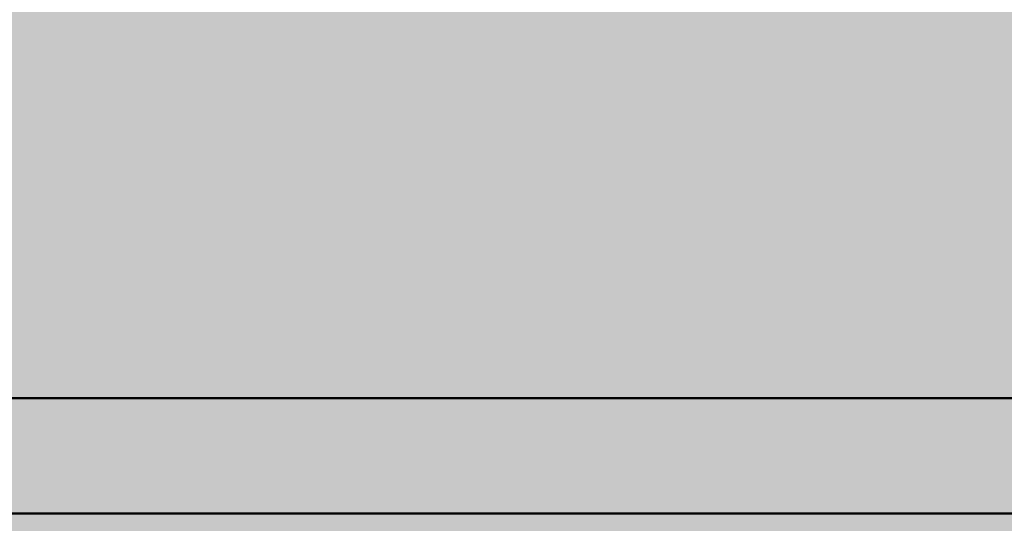
# Model space of a CAD drawing. Units: millimetres. Extents: x 0 to 2267, y 0 to 1823.
# Tile 27 of 256: x 1675 to 1760, y 1117 to 1160. Entities that reach past the tile are written whole.
import ezdxf

# ---------------------------------------------------------------- set-up
doc = ezdxf.new("R2010")
doc.units = ezdxf.units.MM
doc.header["$MEASUREMENT"] = 0
for name, color, linetype, lineweight in [('M-DIMS', 2, 'Continuous', 25), ('M-HATC', 252, 'Continuous', 18), ('M-OUTL', 7, 'Continuous', 50)]:
    doc.layers.add(name, color=color, linetype=linetype, lineweight=lineweight)
doc.styles.get("Standard").update_dxf_attribs({"font": 'arial.ttf'})
doc.dimstyles.get("Standard").update_dxf_attribs({"dimtxt": 7, "dimasz": 4, "dimexe": 0.18, "dimexo": 0.0625, "dimgap": 0.09, "dimtad": 0, "dimdec": 0, "dimzin": 0, "dimdsep": 46, "dimtxsty": 'Standard', "dimcen": 0.09, "dimadec": 0, "dimazin": 0, "dimtfac": 1, "dimtdec": 0, "dimtofl": 0, "dimtmove": 0, "dimatfit": 3, "dimfxl": 1, "dimtolj": 1, "dimtzin": 0, "dimarcsym": 0})

# ---------------------------------------------------------------- blocks, each defined once
blk = doc.blocks.new('*D1')
at = {"layer": 'Defpoints', "color": 0, "transparency": 16777216}
for p in [(1593.429, 1127.417), (1843.429, 1127.417), (1843.429, 955.628)]:
    blk.add_point(p, dxfattribs=at)
at = {"layer": 'M-DIMS', "color": 0, "lineweight": -2, "transparency": 16777216}
for p, q in [((1593.429, 1127.355), (1593.429, 955.448)), ((1843.429, 1127.355), (1843.429, 955.448)), ((1597.429, 955.628), (1710.558, 955.628)), ((1839.429, 955.628), (1726.3, 955.628))]:
    blk.add_line(p, q, dxfattribs=at)
at = {"layer": 'M-DIMS', "color": 0, "transparency": 16777216}
for points in [[(1597.429, 956.294), (1597.429, 954.961), (1593.429, 955.628)], [(1839.429, 956.294), (1839.429, 954.961), (1843.429, 955.628)]]:
    blk.add_solid(points, dxfattribs=at)
at = {"layer": 'M-DIMS', "color": 0, "transparency": 16777216, "insert": (1718.429, 955.628), "char_height": 7, "attachment_point": 5}
blk.add_mtext('\\A1;250', dxfattribs=at)

msp = doc.modelspace()

# ---------------------------------------------------------------- hatches: boundary and pattern name
at = {"layer": 'M-HATC'}
h = msp.add_hatch(color=256, dxfattribs=at)
h.dxf.hatch_style = 1
h.paths.add_polyline_path([(2065.771, 1618.062, 0.236068), (2055.771, 1638.062), (1381.087, 1638.062, 0.236068), (1371.087, 1618.062), (1371.087, 1603.062), (2055.771, 1603.062), (2065.771, 1603.062)])
h.paths.add_polyline_path([(2062.772, 1550.296), (2062.772, 1560.296), (1374.086, 1560.296), (1374.086, 1550.296), (1374.086, 1540.296), (1384.086, 1540.296), (1389.086, 1540.296), (2062.772, 1540.296)])
h.paths.add_polyline_path([(1930.929, 1282.766), (1505.929, 1282.766), (1587.628, 1235.597, 0.131652), (1600.128, 1232.247), (1836.73, 1232.247, 0.131652), (1849.23, 1235.597)])
h.paths.add_polyline_path([(1930.929, 1117.417), (1905.929, 1117.417), (1505.929, 1117.417), (1505.929, 1077.417), (1930.929, 1077.417)])
h = msp.add_hatch(color=256, dxfattribs=at)
h.dxf.hatch_style = 1
h.paths.add_polyline_path([(2055.771, 1603.062), (1381.087, 1603.062), (1381.087, 1598.062), (2055.771, 1598.062)])
h.paths.add_polyline_path([(2055.771, 1598.062), (1381.087, 1598.062), (1381.087, 1593.062), (2055.771, 1593.062)])
h.paths.add_polyline_path([(2051.307, 1536.761), (1385.55, 1536.761), (1385.55, 1526.761), (1387.55, 1526.761), (1388.537, 1525.053), (1385.332, 1521.233), (1385.332, 1521.223), (2050.254, 1522.749), (2048.321, 1525.053), (2049.307, 1526.761), (2051.307, 1526.761)])
edge = h.paths.add_edge_path()
edge.add_arc((1847.535, 1379.149), 135, 222.60306, 222.89085, ccw=False)
edge.add_line((1748.166, 1287.766), (1683.092, 1287.766))
edge.add_arc((1583.724, 1379.149), 135, 317.10915, 317.39694, ccw=False)
edge.add_arc((1678.969, 1290.671), 5, 222.89085, 317.10915, ccw=False)
edge.add_arc((1774.213, 1379.149), 135, 222.60306, 222.89085, ccw=False)
edge.add_line((1674.845, 1287.766), (1609.771, 1287.766))
edge.add_arc((1510.403, 1379.149), 135, 317.10915, 317.39694, ccw=False)
edge.add_arc((1605.647, 1290.671), 5, 222.89085, 317.10915, ccw=False)
edge.add_arc((1700.892, 1379.149), 135, 222.60306, 222.89085, ccw=False)
edge.add_line((1601.524, 1287.766), (1536.45, 1287.766))
edge.add_arc((1437.081, 1379.149), 135, 317.10915, 317.39694, ccw=False)
edge.add_arc((1532.326, 1290.671), 5, 222.89085, 317.10915, ccw=False)
edge.add_arc((1627.571, 1379.149), 135, 222.60306, 222.89085, ccw=False)
edge.add_line((1528.203, 1287.766), (1505.929, 1287.766))
edge.add_spline(control_points=[(1505.929, 1287.766), (1504.262, 1287.766), (1504.262, 1282.766), (1505.929, 1282.766)], knot_values=[0, 0, 0, 0, 5, 5, 5, 5], degree=3, periodic=0)
edge.add_line((1505.929, 1282.766), (1930.929, 1282.766))
edge.add_spline(control_points=[(1930.929, 1282.766), (1932.596, 1282.766), (1932.596, 1287.766), (1930.929, 1287.766)], knot_values=[0, 0, 0, 0, 5, 5, 5, 5], degree=3, periodic=0)
edge.add_line((1930.929, 1287.766), (1903.056, 1287.766))
edge.add_arc((1803.688, 1379.149), 135, 317.10915, 317.39694, ccw=False)
edge.add_arc((1898.932, 1290.671), 5, 222.89085, 317.10915, ccw=False)
edge.add_arc((1994.177, 1379.149), 135, 222.60306, 222.89085, ccw=False)
edge.add_line((1894.809, 1287.766), (1829.735, 1287.766))
edge.add_arc((1730.366, 1379.149), 135, 317.10915, 317.39694, ccw=False)
edge.add_arc((1825.611, 1290.671), 5, 222.89085, 317.10915, ccw=False)
edge.add_arc((1920.856, 1379.149), 135, 222.60306, 222.89085, ccw=False)
edge.add_line((1821.487, 1287.766), (1756.413, 1287.766))
edge.add_arc((1657.045, 1379.149), 135, 317.10915, 317.39694, ccw=False)
edge.add_arc((1752.29, 1290.671), 5, 222.89085, 317.10915, ccw=False)
edge = h.paths.add_edge_path()
edge.add_spline(control_points=[(1843.429, 1227.247), (1845.096, 1227.247), (1845.096, 1232.247), (1843.429, 1232.247)], knot_values=[0, 0, 0, 0, 5, 5, 5, 5], degree=3, periodic=0)
edge.add_line((1843.429, 1232.247), (1593.429, 1232.247))
edge.add_spline(control_points=[(1593.429, 1232.247), (1591.762, 1232.247), (1591.762, 1227.247), (1593.429, 1227.247)], knot_values=[0, 0, 0, 0, 5, 5, 5, 5], degree=3, periodic=0)
edge.add_line((1593.429, 1227.247), (1843.429, 1227.247))
h.paths.add_polyline_path([(1905.929, 1127.417), (1530.929, 1127.417, 0.414214), (1520.929, 1117.417), (1530.929, 1117.417), (1915.929, 1117.417, 0.414214)])
edge = h.paths.add_edge_path()
edge.add_arc((1397.086, 1498.408), 12.73, 90.78215, 190.87871, ccw=False)
edge.add_line((1396.912, 1511.136), (1428.01, 1511.349))
edge.add_line((1428.01, 1511.349), (1433.01, 1511.349))
edge.add_line((1433.01, 1511.349), (1434.439, 1511.349))
edge.add_arc((1419.474, 1498.08), 20, 41.561, 74.08211)
edge.add_line((1424.959, 1517.314), (1399.935, 1517.256))
edge.add_spline(control_points=[(1399.931, 1517.256), (1399.884, 1517.213), (1399.833, 1517.169), (1399.777, 1517.124)], knot_values=[11.567499, 11.567499, 11.567499, 11.567499, 11.814249, 11.814249, 11.814249, 11.814249], degree=3, periodic=0)
edge.add_spline(control_points=[(1399.633, 1517.01), (1399.583, 1516.972), (1399.531, 1516.934), (1399.476, 1516.895)], knot_values=[11.167718, 11.167718, 11.167718, 11.167718, 11.365188, 11.365188, 11.365188, 11.365188], degree=3, periodic=0)
edge.add_spline(control_points=[(1399.34, 1516.8), (1399.151, 1516.672), (1398.938, 1516.538), (1398.704, 1516.399)], knot_values=[10.376405, 10.376405, 10.376405, 10.376405, 11.00994, 11.00994, 11.00994, 11.00994], degree=3, periodic=0)
edge.add_spline(control_points=[(1398.657, 1516.372), (1398.579, 1516.326), (1398.498, 1516.28), (1398.415, 1516.233)], knot_values=[10.125175, 10.125175, 10.125175, 10.125175, 10.334406, 10.334406, 10.334406, 10.334406], degree=3, periodic=0)
edge.add_spline(control_points=[(1398.264, 1516.149), (1398.196, 1516.111), (1398.126, 1516.073), (1398.055, 1516.035)], knot_values=[9.832246, 9.832246, 9.832246, 9.832246, 9.999658, 9.999658, 9.999658, 9.999658], degree=3, periodic=0)
edge.add_spline(control_points=[(1397.999, 1516.005), (1397.731, 1515.862), (1397.446, 1515.717), (1397.147, 1515.571)], knot_values=[9.161808, 9.161808, 9.161808, 9.161808, 9.787769, 9.787769, 9.787769, 9.787769], degree=3, periodic=0)
edge.add_spline(control_points=[(1397.147, 1515.571), (1396.842, 1515.423), (1396.522, 1515.274), (1396.191, 1515.126)], knot_values=[8.524455, 8.524455, 8.524455, 8.524455, 9.161808, 9.161808, 9.161808, 9.161808], degree=3, periodic=0)
edge.add_spline(control_points=[(1396.078, 1515.076), (1395.985, 1515.035), (1395.892, 1514.994), (1395.798, 1514.953)], knot_values=[8.275193, 8.275193, 8.275193, 8.275193, 8.451726, 8.451726, 8.451726, 8.451726], degree=3, periodic=0)
edge.add_spline(control_points=[(1395.602, 1514.869), (1395.5, 1514.826), (1395.397, 1514.782), (1395.293, 1514.739)], knot_values=[7.962917, 7.962917, 7.962917, 7.962917, 8.152764, 8.152764, 8.152764, 8.152764], degree=3, periodic=0)
edge.add_spline(control_points=[(1395.212, 1514.706), (1394.828, 1514.547), (1394.435, 1514.393), (1394.036, 1514.244)], knot_values=[7.21254, 7.21254, 7.21254, 7.21254, 7.913148, 7.913148, 7.913148, 7.913148], degree=3, periodic=0)
edge.add_spline(control_points=[(1394.036, 1514.244), (1393.708, 1514.121), (1393.375, 1514.003), (1393.043, 1513.889)], knot_values=[6.633733, 6.633733, 6.633733, 6.633733, 7.21254, 7.21254, 7.21254, 7.21254], degree=3, periodic=0)
edge.add_spline(control_points=[(1392.821, 1513.815), (1392.72, 1513.781), (1392.618, 1513.748), (1392.517, 1513.715)], knot_values=[6.328796, 6.328796, 6.328796, 6.328796, 6.505493, 6.505493, 6.505493, 6.505493], degree=3, periodic=0)
edge.add_spline(control_points=[(1392.517, 1513.715), (1392.319, 1513.652), (1392.121, 1513.59), (1391.924, 1513.531)], knot_values=[5.984605, 5.984605, 5.984605, 5.984605, 6.328796, 6.328796, 6.328796, 6.328796], degree=3, periodic=0)
edge.add_spline(control_points=[(1391.792, 1513.491), (1391.312, 1513.35), (1390.838, 1513.224), (1390.378, 1513.117)], knot_values=[5.066697, 5.066697, 5.066697, 5.066697, 5.907055, 5.907055, 5.907055, 5.907055], degree=3, periodic=0)
edge.add_spline(control_points=[(1390.378, 1513.117), (1390.18, 1513.071), (1389.984, 1513.028), (1389.791, 1512.99)], knot_values=[4.70367, 4.70367, 4.70367, 4.70367, 5.066695, 5.066695, 5.066695, 5.066695], degree=3, periodic=0)
edge.add_spline(control_points=[(1389.422, 1512.92), (1389.246, 1512.889), (1389.073, 1512.862), (1388.904, 1512.838)], knot_values=[4.130571, 4.130571, 4.130571, 4.130571, 4.469816, 4.469816, 4.469816, 4.469816], degree=3, periodic=0)
edge.add_spline(control_points=[(1388.904, 1512.838), (1388.591, 1512.795), (1388.291, 1512.764), (1388.007, 1512.749)], knot_values=[3.504031, 3.504031, 3.504031, 3.504031, 4.130571, 4.130571, 4.130571, 4.130571], degree=3, periodic=0)
edge.add_spline(control_points=[(1387.936, 1512.746), (1387.854, 1512.742), (1387.773, 1512.74), (1387.694, 1512.739)], knot_values=[3.268866, 3.268866, 3.268866, 3.268866, 3.451164, 3.451164, 3.451164, 3.451164], degree=3, periodic=0)
edge.add_spline(control_points=[(1387.335, 1512.744), (1387.208, 1512.75), (1387.085, 1512.76), (1386.967, 1512.774)], knot_values=[2.670686, 2.670686, 2.670686, 2.670686, 2.984, 2.984, 2.984, 2.984], degree=3, periodic=0)
edge.add_spline(control_points=[(1386.833, 1512.792), (1386.821, 1512.794), (1386.809, 1512.796), (1386.797, 1512.798)], knot_values=[2.516981, 2.516981, 2.516981, 2.516981, 2.549528, 2.549528, 2.549528, 2.549528], degree=3, periodic=0)
edge.add_spline(control_points=[(1386.453, 1512.873), (1386.426, 1512.881), (1386.399, 1512.889), (1386.373, 1512.897)], knot_values=[2.095869, 2.095869, 2.095869, 2.095869, 2.17941, 2.17941, 2.17941, 2.17941], degree=3, periodic=0)
edge.add_spline(control_points=[(1386.069, 1513.019), (1386.063, 1513.022), (1386.058, 1513.025), (1386.052, 1513.028)], knot_values=[1.72453, 1.72453, 1.72453, 1.72453, 1.745933, 1.745933, 1.745933, 1.745933], degree=3, periodic=0)
edge.add_arc((1399.474, 1498.08), 20, 131.82432, 180)
edge.add_arc((1630.334, 1505.548), 250.971, 181.70518, 236.42798)
edge.add_arc((1605.34, 1483.304), 218.782, 238.66083, 243.34961)
edge.add_arc((1647.091, 1510.359), 262.899, 183.12984, 237.85344, ccw=False)
h.paths.add_polyline_path([(1406.537, 1391.964, 0.149382), (1491.551, 1296.442, -0.129517)], flags=17)
edge = h.paths.add_edge_path()
edge.add_arc((2037.384, 1498.08), 20, 0, 48.26587)
edge.add_spline(control_points=[(2050.697, 1513.005), (2050.651, 1512.985), (2050.603, 1512.966), (2050.554, 1512.948)], knot_values=[1.835652, 1.835652, 1.835652, 1.835652, 2.000781, 2.000781, 2.000781, 2.000781], degree=3, periodic=0)
edge.add_spline(control_points=[(2050.462, 1512.917), (2050.479, 1512.922), (2050.496, 1512.928), (2050.513, 1512.934)], knot_values=[2.045477, 2.045477, 2.045477, 2.045477, 2.101389, 2.101389, 2.101389, 2.101389], degree=3, periodic=0)
edge.add_spline(control_points=[(2050.129, 1512.834), (2050.198, 1512.847), (2050.266, 1512.862), (2050.331, 1512.879)], knot_values=[2.237629, 2.237629, 2.237629, 2.237629, 2.435841, 2.435841, 2.435841, 2.435841], degree=3, periodic=0)
edge.add_spline(control_points=[(2050.095, 1512.828), (2050.106, 1512.83), (2050.118, 1512.832), (2050.129, 1512.834)], knot_values=[2.435841, 2.435841, 2.435841, 2.435841, 2.468321, 2.468321, 2.468321, 2.468321], degree=3, periodic=0)
edge.add_spline(control_points=[(2049.784, 1512.785), (2049.855, 1512.792), (2049.924, 1512.801), (2049.992, 1512.811)], knot_values=[2.563852, 2.563852, 2.563852, 2.563852, 2.748541, 2.748541, 2.748541, 2.748541], degree=3, periodic=0)
edge.add_spline(control_points=[(2049.405, 1512.762), (2049.536, 1512.765), (2049.663, 1512.773), (2049.784, 1512.785)], knot_values=[2.748541, 2.748541, 2.748541, 2.748541, 3.064882, 3.064882, 3.064882, 3.064882], degree=3, periodic=0)
edge.add_spline(control_points=[(2049.17, 1512.76), (2049.234, 1512.759), (2049.297, 1512.759), (2049.358, 1512.761)], knot_values=[3.102309, 3.102309, 3.102309, 3.102309, 3.2503, 3.2503, 3.2503, 3.2503], degree=3, periodic=0)
edge.add_spline(control_points=[(2048.857, 1512.769), (2048.964, 1512.764), (2049.068, 1512.761), (2049.17, 1512.76)], knot_values=[3.2503, 3.2503, 3.2503, 3.2503, 3.486069, 3.486069, 3.486069, 3.486069], degree=3, periodic=0)
edge.add_spline(control_points=[(2048.692, 1512.779), (2048.373, 1512.801), (2048.035, 1512.841), (2047.682, 1512.897)], knot_values=[3.606429, 3.606429, 3.606429, 3.606429, 4.2989, 4.2989, 4.2989, 4.2989], degree=3, periodic=0)
edge.add_spline(control_points=[(2047.682, 1512.897), (2047.546, 1512.919), (2047.408, 1512.942), (2047.268, 1512.969)], knot_values=[4.2989, 4.2989, 4.2989, 4.2989, 4.565769, 4.565769, 4.565769, 4.565769], degree=3, periodic=0)
edge.add_spline(control_points=[(2047.268, 1512.969), (2047.145, 1512.991), (2047.021, 1513.016), (2046.895, 1513.042)], knot_values=[4.565769, 4.565769, 4.565769, 4.565769, 4.799971, 4.799971, 4.799971, 4.799971], degree=3, periodic=0)
edge.add_spline(control_points=[(2046.895, 1513.042), (2046.529, 1513.119), (2046.151, 1513.209), (2045.768, 1513.311)], knot_values=[4.799971, 4.799971, 4.799971, 4.799971, 5.483718, 5.483718, 5.483718, 5.483718], degree=3, periodic=0)
edge.add_spline(control_points=[(2045.768, 1513.311), (2045.372, 1513.415), (2044.97, 1513.532), (2044.566, 1513.659)], knot_values=[5.483718, 5.483718, 5.483718, 5.483718, 6.187866, 6.187866, 6.187866, 6.187866], degree=3, periodic=0)
edge.add_spline(control_points=[(2044.566, 1513.659), (2044.415, 1513.706), (2044.263, 1513.755), (2044.112, 1513.805)], knot_values=[6.187866, 6.187866, 6.187866, 6.187866, 6.451551, 6.451551, 6.451551, 6.451551], degree=3, periodic=0)
edge.add_spline(control_points=[(2044.112, 1513.805), (2043.997, 1513.843), (2043.882, 1513.881), (2043.767, 1513.92)], knot_values=[6.451551, 6.451551, 6.451551, 6.451551, 6.651434, 6.651434, 6.651434, 6.651434], degree=3, periodic=0)
edge.add_spline(control_points=[(2043.767, 1513.92), (2043.372, 1514.055), (2042.977, 1514.198), (2042.589, 1514.346)], knot_values=[6.651434, 6.651434, 6.651434, 6.651434, 7.338879, 7.338879, 7.338879, 7.338879], degree=3, periodic=0)
edge.add_spline(control_points=[(2042.589, 1514.346), (2042.164, 1514.507), (2041.746, 1514.675), (2041.341, 1514.846)], knot_values=[7.338879, 7.338879, 7.338879, 7.338879, 8.089209, 8.089209, 8.089209, 8.089209], degree=3, periodic=0)
edge.add_spline(control_points=[(2041.341, 1514.846), (2041.103, 1514.946), (2040.869, 1515.048), (2040.64, 1515.15)], knot_values=[8.089209, 8.089209, 8.089209, 8.089209, 8.529587, 8.529587, 8.529587, 8.529587], degree=3, periodic=0)
edge.add_spline(control_points=[(2040.51, 1515.209), (2040.082, 1515.402), (2039.675, 1515.597), (2039.295, 1515.789)], knot_values=[8.613818, 8.613818, 8.613818, 8.613818, 9.44571, 9.44571, 9.44571, 9.44571], degree=3, periodic=0)
edge.add_spline(control_points=[(2039.295, 1515.789), (2039.062, 1515.907), (2038.839, 1516.025), (2038.629, 1516.14)], knot_values=[9.44571, 9.44571, 9.44571, 9.44571, 9.956404, 9.956404, 9.956404, 9.956404], degree=3, periodic=0)
edge.add_spline(control_points=[(2038.629, 1516.14), (2038.519, 1516.2), (2038.412, 1516.26), (2038.309, 1516.319)], knot_values=[9.956404, 9.956404, 9.956404, 9.956404, 10.223542, 10.223542, 10.223542, 10.223542], degree=3, periodic=0)
edge.add_spline(control_points=[(2038.309, 1516.319), (2038.214, 1516.374), (2038.122, 1516.428), (2038.033, 1516.481)], knot_values=[10.223542, 10.223542, 10.223542, 10.223542, 10.47051, 10.47051, 10.47051, 10.47051], degree=3, periodic=0)
edge.add_spline(control_points=[(2038.033, 1516.481), (2037.786, 1516.63), (2037.564, 1516.773), (2037.372, 1516.909)], knot_values=[10.47051, 10.47051, 10.47051, 10.47051, 11.15767, 11.15767, 11.15767, 11.15767], degree=3, periodic=0)
edge.add_spline(control_points=[(2037.372, 1516.909), (2037.279, 1516.975), (2037.193, 1517.04), (2037.114, 1517.102)], knot_values=[11.15767, 11.15767, 11.15767, 11.15767, 11.49227, 11.49227, 11.49227, 11.49227], degree=3, periodic=0)
edge.add_spline(control_points=[(2036.856, 1517.326), (2036.915, 1517.269), (2036.981, 1517.21), (2037.056, 1517.149)], knot_values=[11.577341, 11.577341, 11.577341, 11.577341, 11.91035, 11.91035, 11.91035, 11.91035], degree=3, periodic=0)
edge.add_spline(control_points=[(2036.807, 1517.375), (2036.823, 1517.359), (2036.839, 1517.342), (2036.856, 1517.326)], knot_values=[11.91035, 11.91035, 11.91035, 11.91035, 12.007402, 12.007402, 12.007402, 12.007402], degree=3, periodic=0)
edge.add_spline(control_points=[(2036.702, 1517.494), (2036.71, 1517.483), (2036.72, 1517.472), (2036.729, 1517.461)], knot_values=[12.184155, 12.184155, 12.184155, 12.184155, 12.255409, 12.255409, 12.255409, 12.255409], degree=3, periodic=0)
edge.add_spline(control_points=[(2036.616, 1517.621), (2036.62, 1517.613), (2036.624, 1517.606), (2036.629, 1517.598)], knot_values=[12.487913, 12.487913, 12.487913, 12.487913, 12.541035, 12.541035, 12.541035, 12.541035], degree=3, periodic=0)
edge.add_spline(control_points=[(2036.563, 1517.786), (2036.564, 1517.779), (2036.564, 1517.773), (2036.565, 1517.766)], knot_values=[12.911761, 12.911761, 12.911761, 12.911761, 12.968286, 12.968286, 12.968286, 12.968286], degree=3, periodic=0)
edge.add_spline(control_points=[(2036.617, 1517.93), (2036.612, 1517.926), (2036.609, 1517.921), (2036.605, 1517.916)], knot_values=[13.382527, 13.382527, 13.382527, 13.382527, 13.433791, 13.433791, 13.433791, 13.433791], degree=3, periodic=0)
edge.add_spline(control_points=[(2036.749, 1518.017), (2036.736, 1518.012), (2036.724, 1518.006), (2036.712, 1518)], knot_values=[13.726299, 13.726299, 13.726299, 13.726299, 13.809928, 13.809928, 13.809928, 13.809928], degree=3, periodic=0)
edge.add_spline(control_points=[(2036.86, 1518.053), (2036.839, 1518.047), (2036.818, 1518.042), (2036.799, 1518.035)], knot_values=[13.910887, 13.910887, 13.910887, 13.910887, 14.02153, 14.02153, 14.02153, 14.02153], degree=3, periodic=0)
edge.add_line((2036.964, 1518.08), (2032.384, 1518.08))
edge.add_line((2032.384, 1518.08), (2027.384, 1518.08))
edge.add_line((2027.384, 1518.08), (2022.384, 1518.08))
edge.add_line((2022.384, 1518.08), (2017.384, 1518.08))
edge.add_arc((2017.384, 1498.08), 20, 90, 138.439)
edge.add_line((2002.419, 1511.349), (2003.848, 1511.349))
edge.add_line((2003.848, 1511.349), (2008.848, 1511.349))
edge.add_line((2008.848, 1511.349), (2039.772, 1511.138))
edge.add_arc((2039.772, 1498.408), 12.73, -10.87871, 90, ccw=False)
edge.add_arc((1789.767, 1510.359), 262.899, 302.14656, 356.87016, ccw=False)
edge.add_arc((1831.518, 1483.304), 218.782, 296.65039, 301.33917)
edge.add_arc((1806.524, 1505.548), 250.971, 303.57202, 358.29482)
h.paths.add_polyline_path([(2030.321, 1391.964, -0.129517), (1945.307, 1296.442, 0.149382)], flags=17)
edge = h.paths.add_edge_path()
edge.add_spline(control_points=[(2037.246, 1518.082), (2037.29, 1518.081), (2037.336, 1518.08), (2037.384, 1518.08)], knot_values=[0.000012, 0.000012, 0.000012, 0.000012, 0.144754, 0.144754, 0.144754, 0.144754], degree=3, periodic=0)
edge.add_line((2037.336, 1518.08), (2037.01, 1518.08))
edge.add_spline(control_points=[(2037.01, 1518.08), (2036.982, 1518.077), (2036.956, 1518.073), (2036.931, 1518.068)], knot_values=[14.13465, 14.13465, 14.13465, 14.13465, 14.247197, 14.247197, 14.247197, 14.247197], degree=3, periodic=0)
edge.add_spline(control_points=[(2036.931, 1518.068), (2036.928, 1518.067), (2036.924, 1518.067), (2036.921, 1518.066)], knot_values=[14.118315, 14.118315, 14.118315, 14.118315, 14.13465, 14.13465, 14.13465, 14.13465], degree=3, periodic=0)
edge.add_spline(control_points=[(2036.921, 1518.066), (2036.912, 1518.064), (2036.903, 1518.063), (2036.895, 1518.061)], knot_values=[14.078086, 14.078086, 14.078086, 14.078086, 14.118315, 14.118315, 14.118315, 14.118315], degree=3, periodic=0)
edge.add_spline(control_points=[(2036.895, 1518.061), (2036.883, 1518.058), (2036.872, 1518.056), (2036.86, 1518.053)], knot_values=[14.02153, 14.02153, 14.02153, 14.02153, 14.078086, 14.078086, 14.078086, 14.078086], degree=3, periodic=0)
edge.add_spline(control_points=[(2036.86, 1518.053), (2036.839, 1518.047), (2036.818, 1518.042), (2036.799, 1518.035)], knot_values=[13.910887, 13.910887, 13.910887, 13.910887, 14.02153, 14.02153, 14.02153, 14.02153], degree=3, periodic=0)
edge.add_spline(control_points=[(2036.799, 1518.035), (2036.798, 1518.035), (2036.797, 1518.035), (2036.797, 1518.035)], knot_values=[13.906906, 13.906906, 13.906906, 13.906906, 13.910887, 13.910887, 13.910887, 13.910887], degree=3, periodic=0)
edge.add_spline(control_points=[(2036.797, 1518.035), (2036.788, 1518.032), (2036.78, 1518.029), (2036.772, 1518.026)], knot_values=[13.857826, 13.857826, 13.857826, 13.857826, 13.906906, 13.906906, 13.906906, 13.906906], degree=3, periodic=0)
edge.add_spline(control_points=[(2036.772, 1518.026), (2036.764, 1518.023), (2036.756, 1518.02), (2036.749, 1518.017)], knot_values=[13.809928, 13.809928, 13.809928, 13.809928, 13.857826, 13.857826, 13.857826, 13.857826], degree=3, periodic=0)
edge.add_spline(control_points=[(2036.749, 1518.017), (2036.736, 1518.012), (2036.724, 1518.006), (2036.712, 1518)], knot_values=[13.726299, 13.726299, 13.726299, 13.726299, 13.809928, 13.809928, 13.809928, 13.809928], degree=3, periodic=0)
edge.add_spline(control_points=[(2036.712, 1518), (2036.712, 1518), (2036.712, 1518), (2036.711, 1518)], knot_values=[13.723993, 13.723993, 13.723993, 13.723993, 13.726299, 13.726299, 13.726299, 13.726299], degree=3, periodic=0)
edge.add_spline(control_points=[(2036.711, 1518), (2036.706, 1517.997), (2036.701, 1517.994), (2036.696, 1517.992)], knot_values=[13.686536, 13.686536, 13.686536, 13.686536, 13.723993, 13.723993, 13.723993, 13.723993], degree=3, periodic=0)
edge.add_spline(control_points=[(2036.696, 1517.992), (2036.692, 1517.989), (2036.687, 1517.987), (2036.683, 1517.984)], knot_values=[13.651251, 13.651251, 13.651251, 13.651251, 13.686536, 13.686536, 13.686536, 13.686536], degree=3, periodic=0)
edge.add_spline(control_points=[(2036.683, 1517.984), (2036.676, 1517.98), (2036.67, 1517.976), (2036.664, 1517.971)], knot_values=[13.596804, 13.596804, 13.596804, 13.596804, 13.651251, 13.651251, 13.651251, 13.651251], degree=3, periodic=0)
edge.add_spline(control_points=[(2036.664, 1517.971), (2036.664, 1517.971), (2036.663, 1517.971), (2036.663, 1517.971)], knot_values=[13.593956, 13.593956, 13.593956, 13.593956, 13.596804, 13.596804, 13.596804, 13.596804], degree=3, periodic=0)
edge.add_spline(control_points=[(2036.663, 1517.971), (2036.66, 1517.969), (2036.658, 1517.967), (2036.655, 1517.965)], knot_values=[13.570322, 13.570322, 13.570322, 13.570322, 13.593956, 13.593956, 13.593956, 13.593956], degree=3, periodic=0)
edge.add_spline(control_points=[(2036.655, 1517.965), (2036.653, 1517.963), (2036.65, 1517.961), (2036.647, 1517.959)], knot_values=[13.545477, 13.545477, 13.545477, 13.545477, 13.570322, 13.570322, 13.570322, 13.570322], degree=3, periodic=0)
edge.add_spline(control_points=[(2036.647, 1517.959), (2036.647, 1517.959), (2036.647, 1517.959), (2036.647, 1517.959)], knot_values=[13.543931, 13.543931, 13.543931, 13.543931, 13.545477, 13.545477, 13.545477, 13.545477], degree=3, periodic=0)
edge.add_spline(control_points=[(2036.647, 1517.959), (2036.641, 1517.954), (2036.636, 1517.949), (2036.631, 1517.945)], knot_values=[13.488237, 13.488237, 13.488237, 13.488237, 13.543931, 13.543931, 13.543931, 13.543931], degree=3, periodic=0)
edge.add_spline(control_points=[(2036.631, 1517.945), (2036.628, 1517.942), (2036.626, 1517.94), (2036.623, 1517.937)], knot_values=[13.460307, 13.460307, 13.460307, 13.460307, 13.488237, 13.488237, 13.488237, 13.488237], degree=3, periodic=0)
edge.add_spline(control_points=[(2036.623, 1517.937), (2036.622, 1517.936), (2036.62, 1517.934), (2036.618, 1517.932)], knot_values=[13.439712, 13.439712, 13.439712, 13.439712, 13.460307, 13.460307, 13.460307, 13.460307], degree=3, periodic=0)
edge.add_spline(control_points=[(2036.618, 1517.932), (2036.618, 1517.931), (2036.617, 1517.931), (2036.617, 1517.93)], knot_values=[13.433791, 13.433791, 13.433791, 13.433791, 13.439712, 13.439712, 13.439712, 13.439712], degree=3, periodic=0)
edge.add_spline(control_points=[(2036.617, 1517.93), (2036.612, 1517.926), (2036.609, 1517.921), (2036.605, 1517.916)], knot_values=[13.382527, 13.382527, 13.382527, 13.382527, 13.433791, 13.433791, 13.433791, 13.433791], degree=3, periodic=0)
edge.add_spline(control_points=[(2036.605, 1517.916), (2036.603, 1517.913), (2036.6, 1517.91), (2036.598, 1517.907)], knot_values=[13.350017, 13.350017, 13.350017, 13.350017, 13.382527, 13.382527, 13.382527, 13.382527], degree=3, periodic=0)
edge.add_spline(control_points=[(2036.598, 1517.907), (2036.597, 1517.906), (2036.596, 1517.904), (2036.595, 1517.903)], knot_values=[13.333922, 13.333922, 13.333922, 13.333922, 13.350017, 13.350017, 13.350017, 13.350017], degree=3, periodic=0)
edge.add_spline(control_points=[(2036.595, 1517.903), (2036.595, 1517.902), (2036.594, 1517.901), (2036.593, 1517.9)], knot_values=[13.323828, 13.323828, 13.323828, 13.323828, 13.333922, 13.333922, 13.333922, 13.333922], degree=3, periodic=0)
edge.add_spline(control_points=[(2036.593, 1517.9), (2036.59, 1517.895), (2036.588, 1517.891), (2036.585, 1517.886)], knot_values=[13.277545, 13.277545, 13.277545, 13.277545, 13.323828, 13.323828, 13.323828, 13.323828], degree=3, periodic=0)
edge.add_spline(control_points=[(2036.585, 1517.886), (2036.584, 1517.883), (2036.582, 1517.879), (2036.58, 1517.875)], knot_values=[13.240119, 13.240119, 13.240119, 13.240119, 13.277545, 13.277545, 13.277545, 13.277545], degree=3, periodic=0)
edge.add_spline(control_points=[(2036.58, 1517.875), (2036.58, 1517.874), (2036.579, 1517.873), (2036.578, 1517.872)], knot_values=[13.228211, 13.228211, 13.228211, 13.228211, 13.240119, 13.240119, 13.240119, 13.240119], degree=3, periodic=0)
edge.add_spline(control_points=[(2036.578, 1517.872), (2036.578, 1517.87), (2036.577, 1517.869), (2036.577, 1517.868)], knot_values=[13.215717, 13.215717, 13.215717, 13.215717, 13.228211, 13.228211, 13.228211, 13.228211], degree=3, periodic=0)
edge.add_spline(control_points=[(2036.577, 1517.868), (2036.575, 1517.864), (2036.574, 1517.86), (2036.573, 1517.857)], knot_values=[13.179847, 13.179847, 13.179847, 13.179847, 13.215717, 13.215717, 13.215717, 13.215717], degree=3, periodic=0)
edge.add_spline(control_points=[(2036.573, 1517.857), (2036.571, 1517.851), (2036.57, 1517.846), (2036.569, 1517.841)], knot_values=[13.132017, 13.132017, 13.132017, 13.132017, 13.179847, 13.179847, 13.179847, 13.179847], degree=3, periodic=0)
edge.add_spline(control_points=[(2036.569, 1517.841), (2036.568, 1517.84), (2036.568, 1517.839), (2036.568, 1517.838)], knot_values=[13.122482, 13.122482, 13.122482, 13.122482, 13.132017, 13.132017, 13.132017, 13.132017], degree=3, periodic=0)
edge.add_spline(control_points=[(2036.568, 1517.838), (2036.568, 1517.836), (2036.567, 1517.835), (2036.567, 1517.833)], knot_values=[13.105592, 13.105592, 13.105592, 13.105592, 13.122482, 13.122482, 13.122482, 13.122482], degree=3, periodic=0)
edge.add_spline(control_points=[(2036.567, 1517.833), (2036.566, 1517.829), (2036.566, 1517.826), (2036.565, 1517.822)], knot_values=[13.074063, 13.074063, 13.074063, 13.074063, 13.105592, 13.105592, 13.105592, 13.105592], degree=3, periodic=0)
edge.add_spline(control_points=[(2036.565, 1517.822), (2036.565, 1517.822), (2036.565, 1517.822), (2036.565, 1517.822)], knot_values=[13.074043, 13.074043, 13.074043, 13.074043, 13.074063, 13.074063, 13.074063, 13.074063], degree=3, periodic=0)
edge.add_spline(control_points=[(2036.565, 1517.822), (2036.564, 1517.816), (2036.564, 1517.811), (2036.564, 1517.805)], knot_values=[13.021884, 13.021884, 13.021884, 13.021884, 13.074043, 13.074043, 13.074043, 13.074043], degree=3, periodic=0)
edge.add_spline(control_points=[(2036.564, 1517.805), (2036.564, 1517.804), (2036.564, 1517.803), (2036.564, 1517.803)], knot_values=[13.01674, 13.01674, 13.01674, 13.01674, 13.021884, 13.021884, 13.021884, 13.021884], degree=3, periodic=0)
edge.add_spline(control_points=[(2036.564, 1517.803), (2036.563, 1517.801), (2036.563, 1517.798), (2036.563, 1517.796)], knot_values=[12.996438, 12.996438, 12.996438, 12.996438, 13.01674, 13.01674, 13.01674, 13.01674], degree=3, periodic=0)
edge.add_spline(control_points=[(2036.563, 1517.796), (2036.563, 1517.793), (2036.563, 1517.789), (2036.563, 1517.786)], knot_values=[12.968286, 12.968286, 12.968286, 12.968286, 12.996438, 12.996438, 12.996438, 12.996438], degree=3, periodic=0)
edge.add_spline(control_points=[(2036.563, 1517.786), (2036.564, 1517.779), (2036.564, 1517.773), (2036.565, 1517.766)], knot_values=[12.911761, 12.911761, 12.911761, 12.911761, 12.968286, 12.968286, 12.968286, 12.968286], degree=3, periodic=0)
edge.add_spline(control_points=[(2036.565, 1517.766), (2036.565, 1517.766), (2036.565, 1517.766), (2036.565, 1517.766)], knot_values=[12.911017, 12.911017, 12.911017, 12.911017, 12.911761, 12.911761, 12.911761, 12.911761], degree=3, periodic=0)
edge.add_spline(control_points=[(2036.565, 1517.766), (2036.565, 1517.762), (2036.566, 1517.759), (2036.566, 1517.756)], knot_values=[12.88528, 12.88528, 12.88528, 12.88528, 12.911017, 12.911017, 12.911017, 12.911017], degree=3, periodic=0)
edge.add_spline(control_points=[(2036.566, 1517.756), (2036.567, 1517.753), (2036.567, 1517.751), (2036.568, 1517.748)], knot_values=[12.862519, 12.862519, 12.862519, 12.862519, 12.88528, 12.88528, 12.88528, 12.88528], degree=3, periodic=0)
edge.add_spline(control_points=[(2036.568, 1517.748), (2036.568, 1517.747), (2036.568, 1517.747), (2036.568, 1517.746)], knot_values=[12.858885, 12.858885, 12.858885, 12.858885, 12.862519, 12.862519, 12.862519, 12.862519], degree=3, periodic=0)
edge.add_spline(control_points=[(2036.568, 1517.746), (2036.569, 1517.74), (2036.571, 1517.733), (2036.572, 1517.726)], knot_values=[12.8053, 12.8053, 12.8053, 12.8053, 12.858885, 12.858885, 12.858885, 12.858885], degree=3, periodic=0)
edge.add_spline(control_points=[(2036.572, 1517.726), (2036.573, 1517.723), (2036.574, 1517.719), (2036.576, 1517.715)], knot_values=[12.775176, 12.775176, 12.775176, 12.775176, 12.8053, 12.8053, 12.8053, 12.8053], degree=3, periodic=0)
edge.add_spline(control_points=[(2036.576, 1517.715), (2036.576, 1517.713), (2036.577, 1517.71), (2036.578, 1517.708)], knot_values=[12.756759, 12.756759, 12.756759, 12.756759, 12.775176, 12.775176, 12.775176, 12.775176], degree=3, periodic=0)
edge.add_spline(control_points=[(2036.578, 1517.708), (2036.578, 1517.707), (2036.578, 1517.706), (2036.579, 1517.705)], knot_values=[12.748742, 12.748742, 12.748742, 12.748742, 12.756759, 12.756759, 12.756759, 12.756759], degree=3, periodic=0)
edge.add_spline(control_points=[(2036.579, 1517.705), (2036.581, 1517.698), (2036.583, 1517.692), (2036.586, 1517.685)], knot_values=[12.69959, 12.69959, 12.69959, 12.69959, 12.748742, 12.748742, 12.748742, 12.748742], degree=3, periodic=0)
edge.add_spline(control_points=[(2036.586, 1517.685), (2036.588, 1517.68), (2036.59, 1517.675), (2036.592, 1517.669)], knot_values=[12.659038, 12.659038, 12.659038, 12.659038, 12.69959, 12.69959, 12.69959, 12.69959], degree=3, periodic=0)
edge.add_spline(control_points=[(2036.592, 1517.669), (2036.594, 1517.665), (2036.596, 1517.66), (2036.598, 1517.656)], knot_values=[12.626806, 12.626806, 12.626806, 12.626806, 12.659038, 12.659038, 12.659038, 12.659038], degree=3, periodic=0)
edge.add_spline(control_points=[(2036.598, 1517.656), (2036.598, 1517.655), (2036.599, 1517.654), (2036.599, 1517.653)], knot_values=[12.619394, 12.619394, 12.619394, 12.619394, 12.626806, 12.626806, 12.626806, 12.626806], degree=3, periodic=0)
edge.add_spline(control_points=[(2036.599, 1517.653), (2036.604, 1517.642), (2036.61, 1517.632), (2036.616, 1517.621)], knot_values=[12.541039, 12.541039, 12.541039, 12.541039, 12.619394, 12.619394, 12.619394, 12.619394], degree=3, periodic=0)
edge.add_spline(control_points=[(2036.616, 1517.621), (2036.616, 1517.621), (2036.616, 1517.621), (2036.616, 1517.621)], knot_values=[12.541035, 12.541035, 12.541035, 12.541035, 12.541039, 12.541039, 12.541039, 12.541039], degree=3, periodic=0)
edge.add_spline(control_points=[(2036.616, 1517.621), (2036.62, 1517.613), (2036.624, 1517.606), (2036.629, 1517.598)], knot_values=[12.487913, 12.487913, 12.487913, 12.487913, 12.541035, 12.541035, 12.541035, 12.541035], degree=3, periodic=0)
edge.add_spline(control_points=[(2036.629, 1517.598), (2036.633, 1517.592), (2036.637, 1517.585), (2036.641, 1517.579)], knot_values=[12.443982, 12.443982, 12.443982, 12.443982, 12.487913, 12.487913, 12.487913, 12.487913], degree=3, periodic=0)
edge.add_spline(control_points=[(2036.641, 1517.579), (2036.641, 1517.578), (2036.642, 1517.576), (2036.643, 1517.575)], knot_values=[12.434996, 12.434996, 12.434996, 12.434996, 12.443982, 12.443982, 12.443982, 12.443982], degree=3, periodic=0)
edge.add_spline(control_points=[(2036.643, 1517.575), (2036.653, 1517.56), (2036.664, 1517.544), (2036.676, 1517.528)], knot_values=[12.329647, 12.329647, 12.329647, 12.329647, 12.434996, 12.434996, 12.434996, 12.434996], degree=3, periodic=0)
edge.add_spline(control_points=[(2036.676, 1517.528), (2036.684, 1517.517), (2036.693, 1517.505), (2036.702, 1517.494)], knot_values=[12.255409, 12.255409, 12.255409, 12.255409, 12.329647, 12.329647, 12.329647, 12.329647], degree=3, periodic=0)
edge.add_spline(control_points=[(2036.702, 1517.494), (2036.71, 1517.483), (2036.72, 1517.472), (2036.729, 1517.461)], knot_values=[12.184155, 12.184155, 12.184155, 12.184155, 12.255409, 12.255409, 12.255409, 12.255409], degree=3, periodic=0)
edge.add_spline(control_points=[(2036.729, 1517.461), (2036.744, 1517.444), (2036.759, 1517.426), (2036.775, 1517.409)], knot_values=[12.075961, 12.075961, 12.075961, 12.075961, 12.184155, 12.184155, 12.184155, 12.184155], degree=3, periodic=0)
edge.add_spline(control_points=[(2036.775, 1517.409), (2036.776, 1517.407), (2036.777, 1517.406), (2036.778, 1517.405)], knot_values=[12.069502, 12.069502, 12.069502, 12.069502, 12.075961, 12.075961, 12.075961, 12.075961], degree=3, periodic=0)
edge.add_spline(control_points=[(2036.778, 1517.405), (2036.788, 1517.395), (2036.797, 1517.385), (2036.807, 1517.375)], knot_values=[12.007402, 12.007402, 12.007402, 12.007402, 12.069502, 12.069502, 12.069502, 12.069502], degree=3, periodic=0)
edge.add_spline(control_points=[(2036.807, 1517.375), (2036.823, 1517.359), (2036.839, 1517.342), (2036.856, 1517.326)], knot_values=[11.91035, 11.91035, 11.91035, 11.91035, 12.007402, 12.007402, 12.007402, 12.007402], degree=3, periodic=0)
edge.add_spline(control_points=[(2036.856, 1517.326), (2036.915, 1517.269), (2036.981, 1517.21), (2037.056, 1517.149)], knot_values=[11.577341, 11.577341, 11.577341, 11.577341, 11.91035, 11.91035, 11.91035, 11.91035], degree=3, periodic=0)
edge.add_spline(control_points=[(2037.056, 1517.149), (2037.075, 1517.134), (2037.094, 1517.118), (2037.114, 1517.102)], knot_values=[11.49227, 11.49227, 11.49227, 11.49227, 11.577341, 11.577341, 11.577341, 11.577341], degree=3, periodic=0)
edge.add_spline(control_points=[(2037.114, 1517.102), (2037.193, 1517.04), (2037.279, 1516.975), (2037.372, 1516.909)], knot_values=[11.15767, 11.15767, 11.15767, 11.15767, 11.49227, 11.49227, 11.49227, 11.49227], degree=3, periodic=0)
edge.add_spline(control_points=[(2037.372, 1516.909), (2037.564, 1516.773), (2037.786, 1516.63), (2038.033, 1516.481)], knot_values=[10.47051, 10.47051, 10.47051, 10.47051, 11.15767, 11.15767, 11.15767, 11.15767], degree=3, periodic=0)
edge.add_spline(control_points=[(2038.033, 1516.481), (2038.122, 1516.428), (2038.214, 1516.374), (2038.309, 1516.319)], knot_values=[10.223542, 10.223542, 10.223542, 10.223542, 10.47051, 10.47051, 10.47051, 10.47051], degree=3, periodic=0)
edge.add_spline(control_points=[(2038.309, 1516.319), (2038.412, 1516.26), (2038.519, 1516.2), (2038.629, 1516.14)], knot_values=[9.956404, 9.956404, 9.956404, 9.956404, 10.223542, 10.223542, 10.223542, 10.223542], degree=3, periodic=0)
edge.add_spline(control_points=[(2038.629, 1516.14), (2038.839, 1516.025), (2039.062, 1515.907), (2039.295, 1515.789)], knot_values=[9.44571, 9.44571, 9.44571, 9.44571, 9.956404, 9.956404, 9.956404, 9.956404], degree=3, periodic=0)
edge.add_spline(control_points=[(2039.295, 1515.789), (2039.675, 1515.597), (2040.082, 1515.402), (2040.51, 1515.209)], knot_values=[8.613818, 8.613818, 8.613818, 8.613818, 9.44571, 9.44571, 9.44571, 9.44571], degree=3, periodic=0)
edge.add_spline(control_points=[(2040.51, 1515.209), (2040.553, 1515.189), (2040.597, 1515.17), (2040.64, 1515.15)], knot_values=[8.529587, 8.529587, 8.529587, 8.529587, 8.613818, 8.613818, 8.613818, 8.613818], degree=3, periodic=0)
edge.add_spline(control_points=[(2040.64, 1515.15), (2040.869, 1515.048), (2041.103, 1514.946), (2041.341, 1514.846)], knot_values=[8.089209, 8.089209, 8.089209, 8.089209, 8.529587, 8.529587, 8.529587, 8.529587], degree=3, periodic=0)
edge.add_spline(control_points=[(2041.341, 1514.846), (2041.746, 1514.675), (2042.164, 1514.507), (2042.589, 1514.346)], knot_values=[7.338879, 7.338879, 7.338879, 7.338879, 8.089209, 8.089209, 8.089209, 8.089209], degree=3, periodic=0)
edge.add_spline(control_points=[(2042.589, 1514.346), (2042.977, 1514.198), (2043.372, 1514.055), (2043.767, 1513.92)], knot_values=[6.651434, 6.651434, 6.651434, 6.651434, 7.338879, 7.338879, 7.338879, 7.338879], degree=3, periodic=0)
edge.add_spline(control_points=[(2043.767, 1513.92), (2043.882, 1513.881), (2043.997, 1513.843), (2044.112, 1513.805)], knot_values=[6.451551, 6.451551, 6.451551, 6.451551, 6.651434, 6.651434, 6.651434, 6.651434], degree=3, periodic=0)
edge.add_spline(control_points=[(2044.112, 1513.805), (2044.263, 1513.755), (2044.415, 1513.706), (2044.566, 1513.659)], knot_values=[6.187866, 6.187866, 6.187866, 6.187866, 6.451551, 6.451551, 6.451551, 6.451551], degree=3, periodic=0)
edge.add_spline(control_points=[(2044.566, 1513.659), (2044.97, 1513.532), (2045.372, 1513.415), (2045.768, 1513.311)], knot_values=[5.483718, 5.483718, 5.483718, 5.483718, 6.187866, 6.187866, 6.187866, 6.187866], degree=3, periodic=0)
edge.add_spline(control_points=[(2045.768, 1513.311), (2046.151, 1513.209), (2046.529, 1513.119), (2046.895, 1513.042)], knot_values=[4.799971, 4.799971, 4.799971, 4.799971, 5.483718, 5.483718, 5.483718, 5.483718], degree=3, periodic=0)
edge.add_spline(control_points=[(2046.895, 1513.042), (2047.021, 1513.016), (2047.145, 1512.991), (2047.268, 1512.969)], knot_values=[4.565769, 4.565769, 4.565769, 4.565769, 4.799971, 4.799971, 4.799971, 4.799971], degree=3, periodic=0)
edge.add_spline(control_points=[(2047.268, 1512.969), (2047.408, 1512.942), (2047.546, 1512.919), (2047.682, 1512.897)], knot_values=[4.2989, 4.2989, 4.2989, 4.2989, 4.565769, 4.565769, 4.565769, 4.565769], degree=3, periodic=0)
edge.add_spline(control_points=[(2047.682, 1512.897), (2048.035, 1512.841), (2048.373, 1512.801), (2048.692, 1512.779)], knot_values=[3.606429, 3.606429, 3.606429, 3.606429, 4.2989, 4.2989, 4.2989, 4.2989], degree=3, periodic=0)
edge.add_spline(control_points=[(2048.692, 1512.779), (2048.748, 1512.775), (2048.803, 1512.772), (2048.857, 1512.769)], knot_values=[3.486069, 3.486069, 3.486069, 3.486069, 3.606429, 3.606429, 3.606429, 3.606429], degree=3, periodic=0)
edge.add_spline(control_points=[(2048.857, 1512.769), (2048.964, 1512.764), (2049.068, 1512.761), (2049.17, 1512.76)], knot_values=[3.2503, 3.2503, 3.2503, 3.2503, 3.486069, 3.486069, 3.486069, 3.486069], degree=3, periodic=0)
edge.add_spline(control_points=[(2049.17, 1512.76), (2049.234, 1512.759), (2049.297, 1512.759), (2049.358, 1512.761)], knot_values=[3.102309, 3.102309, 3.102309, 3.102309, 3.2503, 3.2503, 3.2503, 3.2503], degree=3, periodic=0)
edge.add_spline(control_points=[(2049.358, 1512.761), (2049.374, 1512.761), (2049.39, 1512.761), (2049.405, 1512.762)], knot_values=[3.064882, 3.064882, 3.064882, 3.064882, 3.102309, 3.102309, 3.102309, 3.102309], degree=3, periodic=0)
edge.add_spline(control_points=[(2049.405, 1512.762), (2049.536, 1512.765), (2049.663, 1512.773), (2049.784, 1512.785)], knot_values=[2.748541, 2.748541, 2.748541, 2.748541, 3.064882, 3.064882, 3.064882, 3.064882], degree=3, periodic=0)
edge.add_spline(control_points=[(2049.784, 1512.785), (2049.855, 1512.792), (2049.924, 1512.801), (2049.992, 1512.811)], knot_values=[2.563852, 2.563852, 2.563852, 2.563852, 2.748541, 2.748541, 2.748541, 2.748541], degree=3, periodic=0)
edge.add_spline(control_points=[(2049.992, 1512.811), (2050.026, 1512.816), (2050.061, 1512.822), (2050.095, 1512.828)], knot_values=[2.468321, 2.468321, 2.468321, 2.468321, 2.563852, 2.563852, 2.563852, 2.563852], degree=3, periodic=0)
edge.add_spline(control_points=[(2050.095, 1512.828), (2050.106, 1512.83), (2050.118, 1512.832), (2050.129, 1512.834)], knot_values=[2.435841, 2.435841, 2.435841, 2.435841, 2.468321, 2.468321, 2.468321, 2.468321], degree=3, periodic=0)
edge.add_spline(control_points=[(2050.129, 1512.834), (2050.198, 1512.847), (2050.266, 1512.862), (2050.331, 1512.879)], knot_values=[2.237629, 2.237629, 2.237629, 2.237629, 2.435841, 2.435841, 2.435841, 2.435841], degree=3, periodic=0)
edge.add_spline(control_points=[(2050.331, 1512.879), (2050.375, 1512.891), (2050.419, 1512.903), (2050.462, 1512.917)], knot_values=[2.101389, 2.101389, 2.101389, 2.101389, 2.237629, 2.237629, 2.237629, 2.237629], degree=3, periodic=0)
edge.add_spline(control_points=[(2050.462, 1512.917), (2050.479, 1512.922), (2050.496, 1512.928), (2050.513, 1512.934)], knot_values=[2.045477, 2.045477, 2.045477, 2.045477, 2.101389, 2.101389, 2.101389, 2.101389], degree=3, periodic=0)
edge.add_spline(control_points=[(2050.513, 1512.934), (2050.527, 1512.938), (2050.54, 1512.943), (2050.554, 1512.948)], knot_values=[2.000781, 2.000781, 2.000781, 2.000781, 2.045477, 2.045477, 2.045477, 2.045477], degree=3, periodic=0)
edge.add_spline(control_points=[(2050.554, 1512.948), (2050.603, 1512.966), (2050.651, 1512.985), (2050.697, 1513.005)], knot_values=[1.835652, 1.835652, 1.835652, 1.835652, 2.000781, 2.000781, 2.000781, 2.000781], degree=3, periodic=0)
edge.add_arc((2037.384, 1498.08), 20, 48.26587, 90.12993)
edge = h.paths.add_edge_path(flags=16)
edge.add_spline(control_points=[(1386.139, 1512.986), (1388.92, 1511.739), (1398.039, 1515.519), (1399.931, 1517.256)], knot_values=[1.831046, 1.831046, 1.831046, 1.831046, 11.814249, 11.814249, 11.814249, 11.814249], degree=3, periodic=0)
edge.add_line((1399.931, 1517.256), (1393.743, 1517.242))
edge.add_arc((1399.474, 1498.08), 20, 106.6501, 131.8173)
h = msp.add_hatch(color=256, dxfattribs=at)
h.dxf.hatch_style = 1
h.paths.add_polyline_path([(2042.889, 1580.18), (2055.771, 1593.062), (1381.087, 1593.062), (1393.969, 1580.18), (1374.086, 1560.296), (2062.772, 1560.296)])
h.paths.add_polyline_path([(1843.429, 1201.33), (1843.429, 1227.247), (1593.429, 1227.247), (1593.429, 1201.33, -0.228274), (1574.599, 1162.235), (1530.929, 1127.417), (1905.929, 1127.417), (1862.259, 1162.235, -0.228274)])

# ---------------------------------------------------------------- linework, layer by layer
at = {"layer": 'M-OUTL'}
for p, q in [((1530.929, 1127.417), (1905.929, 1127.417)), ((1505.929, 1117.417), (1930.929, 1117.417)), ((1718.429, 1117.417), (1593.429, 1117.417)), ((1718.429, 1117.417), (1843.429, 1117.417))]:
    msp.add_line(p, q, dxfattribs=at)

# ---------------------------------------------------------------- dimensions: what is measured, and where the dimension line sits
at = {"layer": 'M-DIMS'}
dim = msp.add_linear_dim(base=(1843.429, 955.628), p1=(1593.429, 1127.417), p2=(1843.429, 1127.417), dimstyle='Standard', override={"dimclrd": 0, "dimclre": 0, "dimclrt": 0}, dxfattribs=at)
dim.commit()
dim.dimension.update_dxf_attribs({"geometry": '*D1', "text_midpoint": (1718.429, 955.628)})

doc.saveas('drawing.dxf')
